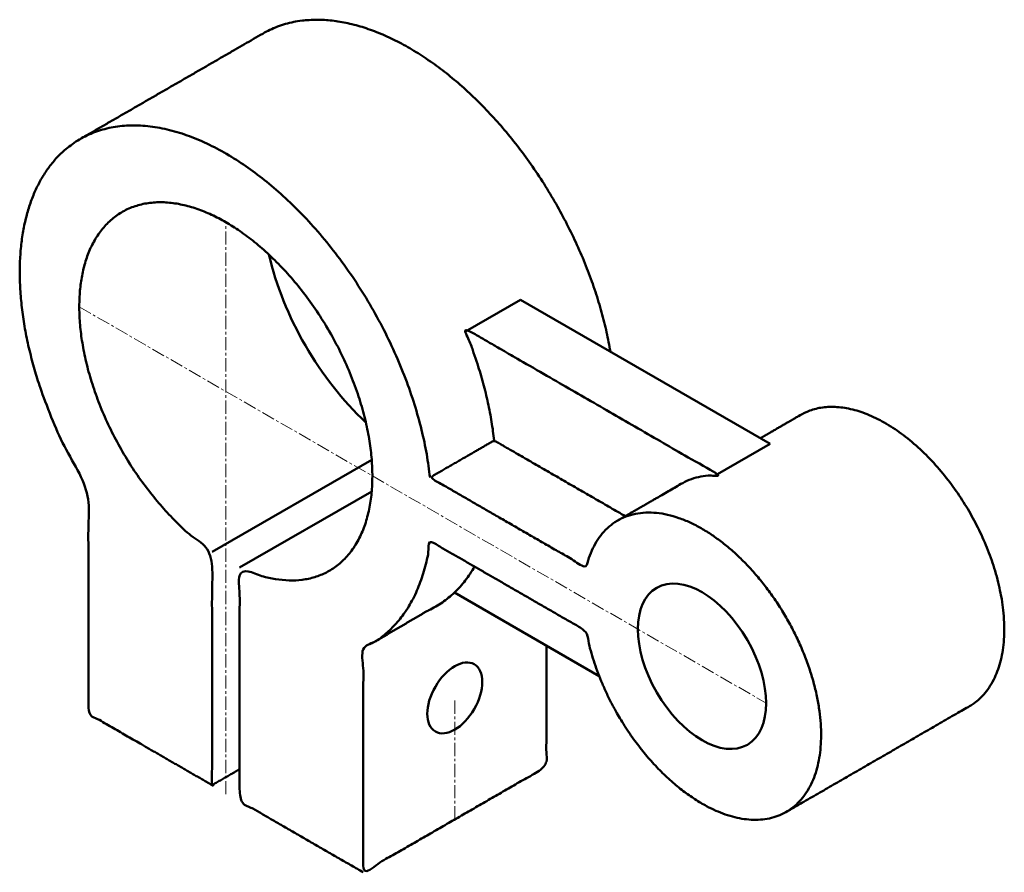
# Model space of a CAD drawing. Units: millimetres. Extents: x -6.5 to 86.7, y 47.5 to 128.2.
import ezdxf

# ---------------------------------------------------------------- set-up
doc = ezdxf.new("R2010")
doc.units = ezdxf.units.MM
doc.header["$MEASUREMENT"] = 0
doc.linetypes.add('CENTER', pattern=[2, 1.25, -0.25, 0.25, -0.25])
doc.layers.add('M-CNTR', color=4, linetype='CENTER', lineweight=18)
doc.layers.add('M-OUTL', color=7, linetype='Continuous', lineweight=50)

msp = doc.modelspace()

# ---------------------------------------------------------------- linework, layer by layer
at = {"layer": 'M-CNTR'}
for p, q in [((13.037, 54.878), (13.037, 108.998)), ((-0.82, 100.998), (64.132, 63.498)), ((34.687, 52.498), (34.687, 63.998))]:
    msp.add_line(p, q, dxfattribs=at)
at = {"layer": 'M-OUTL'}
for p, q in [((35.716, 98.654), (40.912, 101.654)), ((64.512, 88.029), (40.912, 101.654)), ((59.315, 85.029), (64.511, 88.029)), ((11.737, 77.818), (26.832, 86.533)), ((14.335, 76.318), (26.832, 83.533)), ((34.655, 73.967), (48.345, 66.062))]:
    msp.add_line(p, q, dxfattribs=at)
msp.add_ellipse((30.357, 102.998), major_axis=(9.798, -16.971), ratio=0.57735, start_param=10.508879, end_param=11.482269, dxfattribs=at)
for centre, major_axis in [((58.07, 66.998), (4.287, -7.425)), ((34.687, 63.998), (-1.837, -3.182))]:
    msp.add_ellipse(centre, major_axis=major_axis, ratio=0.57735, dxfattribs=at)
for points, weights, knots in [([(49.403, 96.752), (46.961, 111.222), (35.861, 121.405), (24.761, 131.587), (16.579, 126.863), (7.919, 121.863), (-0.742, 116.863)], [1, 0.859826965317, 1, 0.859826965317, 1, 1, 1], [0, 0, 0, 1.071731, 1.071731, 2.143463, 2.143463, 3.143463, 3.143463, 3.143463]), ([(32.348, 84.848), (30.408, 102.623), (16.027, 113.505), (1.647, 124.387), (-4.577, 112.79), (-10.801, 101.193), (0.046, 83.727), (0.046, 73.113), (0.046, 62.498), (5.892, 59.123), (11.738, 55.748)], [1, 0.801206070409, 1, 0.801206070409, 1, 0.801206070409, 1, 1, 1, 1, 1], [0, 0, 0, 1.282977, 1.282977, 2.565953, 2.565953, 3.84893, 3.84893, 4.84893, 4.84893, 5.84893, 5.84893, 5.84893]), ([(26.027, 47.498), (20.181, 50.873), (14.336, 54.248), (14.336, 65.283), (14.336, 76.318), (27.498, 70.15), (26.878, 85.758), (26.257, 101.365), (13.037, 108.998), (-0.184, 116.631), (-0.804, 101.74), (-1.425, 86.849), (11.738, 77.818), (11.738, 66.783), (11.738, 55.748), (13.037, 56.498), (14.336, 57.248)], [1, 1, 1, 1, 1, 0.723507670128, 1, 0.723507670128, 1, 0.723507670128, 1, 0.723507670128, 1, 1, 1, 1, 1], [0, 0, 0, 1, 1, 2, 2, 3.523852, 3.523852, 5.047705, 5.047705, 6.571557, 6.571557, 8.09541, 8.09541, 9.09541, 9.09541, 10.09541, 10.09541, 10.09541]), ([(38.41, 88.348), (37.845, 93.531), (35.582, 98.982), (47.692, 91.99), (59.802, 84.998), (57.746, 85.196), (56.171, 84.287), (53.14, 82.537), (50.109, 80.787)], [1, 0.977103731582, 1, 1, 1, 0.980988811984, 1, 1, 1], [0, 0, 0, 0.428805, 0.428805, 1.428805, 1.428805, 1.819412, 1.819412, 2.819412, 2.819412, 2.819412]), ([(66.031, 53.209), (74.691, 58.209), (83.351, 63.209), (91.312, 67.806), (83.351, 81.594), (75.39, 95.383), (67.43, 90.787), (65.506, 89.676), (63.583, 88.566)], [1, 1, 1, 0.707106781187, 1, 0.707106781187, 1, 1, 1], [0, 0, 0, 1, 1, 2.570796, 2.570796, 4.141593, 4.141593, 5.141593, 5.141593, 5.141593]), ([(43.348, 68.948), (43.348, 63.223), (43.348, 57.498), (34.687, 52.498), (26.027, 47.498), (26.027, 58.113), (26.027, 68.727), (31.389, 71.17), (32.348, 78.848), (39.732, 74.585), (47.116, 70.323), (49.427, 57.732), (59.378, 53.331), (69.328, 48.93), (69.328, 60.498), (69.328, 72.066), (59.378, 79.155), (49.427, 86.244), (47.116, 76.323), (39.732, 80.585), (32.348, 84.848), (35.379, 86.598), (38.41, 88.348), (44.609, 84.769), (50.809, 81.19)], [1, 1, 1, 1, 1, 1, 1, 0.938108460027, 1, 1, 1, 0.7470512655, 1, 0.7470512655, 1, 0.7470512655, 1, 0.7470512655, 1, 1, 1, 1, 1, 1, 1], [0, 0, 0, 1, 1, 2, 2, 3, 3, 3.707337, 3.707337, 4.707337, 4.707337, 6.161699, 6.161699, 7.616062, 7.616062, 9.070424, 9.070424, 10.524786, 10.524786, 11.524786, 11.524786, 12.524786, 12.524786, 13.524786, 13.524786, 13.524786]), ([(26.815, 69.133), (29.452, 70.68), (32.089, 72.227), (34.886, 73.501), (36.554, 76.42)], [1, 1, 1, 0.981955601759, 1], [0, 0, 0, 1, 1, 1.380515, 1.380515, 1.380515])]:
    msp.add_rational_spline(points, weights, degree=2, knots=knots, dxfattribs=at)

doc.saveas('drawing.dxf')
